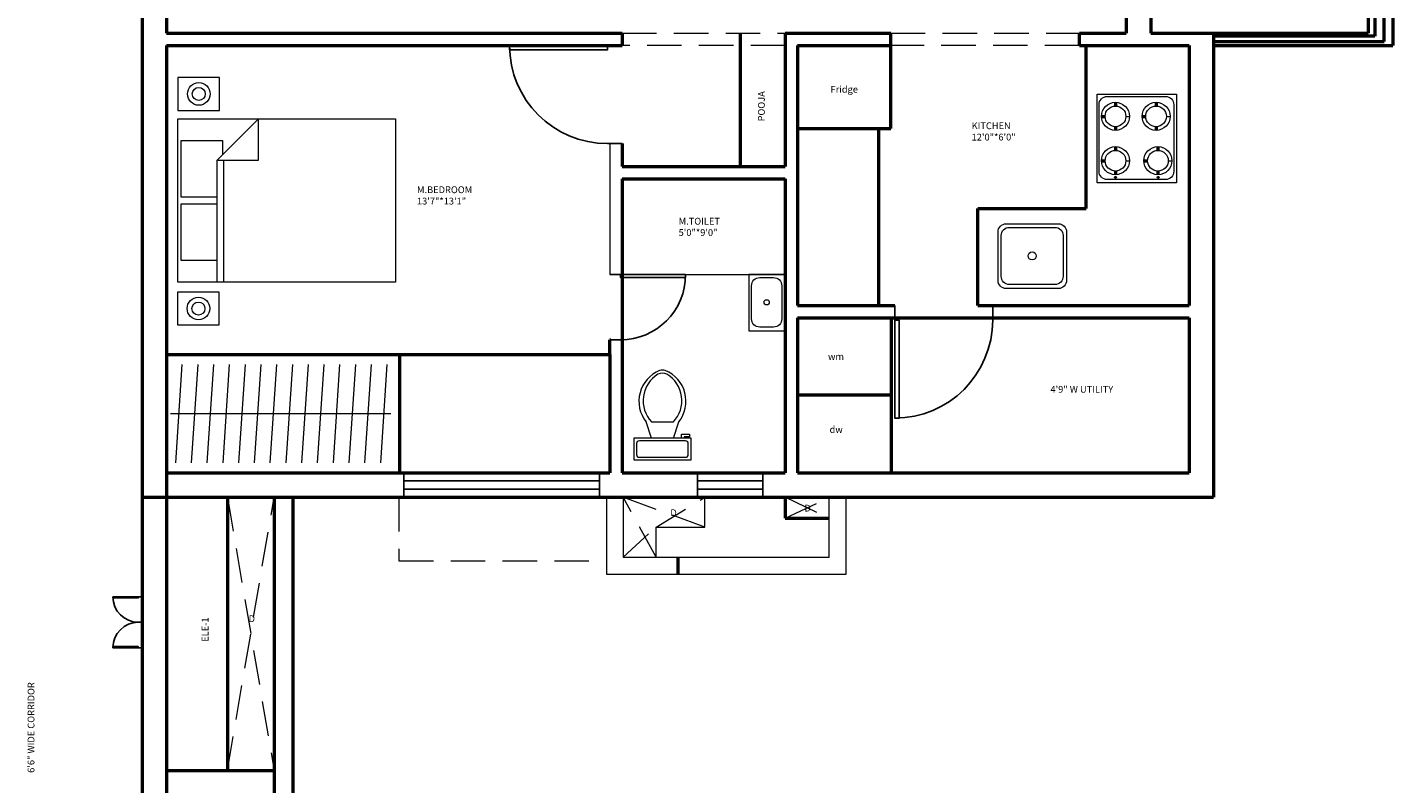
# Model space of a CAD drawing. Units: inches. Extents: x 4795 to 6024, y 2716 to 5025.
# Tile 15 of 19: x 5486 to 5988, y 3816 to 4094. Entities that reach past the tile are written whole.
import ezdxf

# ---------------------------------------------------------------- set-up
doc = ezdxf.new("R2010")
doc.units = ezdxf.units.IN
doc.linetypes.add('DASHED', pattern=[19.05, 12.7, -6.35])
for name, color, linetype, lineweight in [('A-ANNO-TEXT', 7, 'Continuous', 18), ('A-AREA-IDEN', 3, 'Continuous', 18), ('A-DOOR', 4, 'Continuous', 25), ('A-FLOR-FIXT', 9, 'Continuous', 18), ('A-FURN', 8, 'Continuous', 18), ('A-GLAZ', 4, 'Continuous', 25), ('A-WALL', 7, 'Continuous', 50), ('A-WALL-OVHD', 8, 'DASHED', 18)]:
    doc.layers.add(name, color=color, linetype=linetype, lineweight=lineweight)
doc.styles.get("Standard").update_dxf_attribs({"font": 'arial.ttf'})

# ---------------------------------------------------------------- blocks, each defined once
blk = doc.blocks.new('*U2')
for p, q in [((0, 0), (0, -6)), ((40, 0), (40, -6))]:
    blk.add_line(p, q)
blk.add_lwpolyline([(0, 0), (0, 40), (1.75, 40), (1.75, 0)], close=True)
blk.add_arc((0, 0), 40, 0, 90)
blk = doc.blocks.new('Bed - Queen')
for p, q in [((0, -80.00003), (0, 0)), ((0, 0), (59.99999, 0)), ((59.99999, 0), (59.99999, -80.00003)), ((7.99999, -1.2), (28.79998, -1.2)), ((7.99999, -14.4), (7.99999, -1.2)), ((28.79998, -1.2), (28.79998, -14.4)), ((31.19999, -1.2), (51.99999, -1.2)), ((31.19999, -14.4), (31.19999, -1.2)), ((51.99999, -1.2), (51.99999, -16.4)), ((0, -14.4), (44.8, -14.4)), ((59.99999, -29.6), (44.8, -14.4)), ((44.8, -14.4), (44.8, -29.6)), ((44.8, -16.8), (0, -16.8)), ((51.99999, -16.4), (46.79936, -16.4)), ((44.8, -29.6), (59.99999, -29.6)), ((59.99999, -80.00003), (0, -80.00003))]:
    blk.add_line(p, q)
blk = doc.blocks.new('Toilet - top')
for p, q in [((9.5, -6), (9.5, -2)), ((-10, -8.5), (-8, -8.5)), ((-10, -9.5), (-10, -8.5)), ((-7, -9.5), (-10, -9.5)), ((-8, -8.5), (-8, -8)), ((-7, -8), (-7, -9.5)), ((-4, -8), (-6, -14)), ((4, -8), (6, -14)), ((4, -14), (-4, -14))]:
    blk.add_line(p, q)
blk.add_lwpolyline([(10.5, -8), (10.5, 0), (-10.5, 0), (-10.5, -8)], close=True)
for points in [[(-9.5, -2), (-9.5, -6)], [(8.5, -1), (-8.5, -1)], [(-8.5, -7), (8.5, -7)]]:
    blk.add_lwpolyline(points)
for centre, radius, start, end in [((-8.62, -1.88), 0.884, 81.8699, 188.1301), ((8.62, -1.88), 0.884, 351.8699, 98.1301), ((-8.62, -6.12), 0.884, 171.8699, 278.1301), ((8.62, -6.12), 0.884, 261.8699, 8.1301), ((3.52, -21.58), 12.17, 141.4691, 247.9714), ((4.2, -21.82), 11.33, 136.3677, 238.9468), ((-3.52, -21.58), 12.17, 292.0284, 38.5307), ((-4.2, -21.82), 11.33, 301.053, 43.6321), ((0, -27.88), 4, 245.7318, 294.2682), ((0, -29), 4, 254.8605, 285.1395)]:
    blk.add_arc(centre, radius, start, end)
blk = doc.blocks.new('WIN-72')
for p, q in [((0, 0), (0, 9)), ((0, 9), (72, 9)), ((0, 6), (72, 6)), ((72, 9), (72, 0)), ((72, 3), (0, 3)), ((72, 0), (0, 0))]:
    blk.add_line(p, q)
blk = doc.blocks.new('WIN-24')
for p, q in [((0, 0), (0, 9)), ((0, 9), (24, 9)), ((0, 6), (24, 6)), ((24, 9), (24, 0)), ((24, 3), (0, 3)), ((24, 0), (0, 0))]:
    blk.add_line(p, q)

msp = doc.modelspace()

# ---------------------------------------------------------------- linework, layer by layer
at = {"layer": 'A-FLOR-FIXT'}
for points in [[(5879.38, 4068.91), (5908.62, 4068.91), (5908.62, 4036.39), (5879.38, 4036.39)], [(5764.72, 4002.66), (5751.28, 4002.66), (5751.28, 3981.93), (5764.72, 3981.93)]]:
    msp.add_lwpolyline(points, close=True, dxfattribs=at)
for points in [[(5883.1, 4068.11), (5904.57, 4068.11, -0.414214), (5907.57, 4065.11), (5907.57, 4040.56, -0.414214), (5904.57, 4037.56), (5883.1, 4037.56, -0.414214), (5880.1, 4040.56), (5880.1, 4065.11, -0.414214)], [(5845.95, 4021.32), (5865.16, 4021.32, -0.414214), (5868.16, 4018.32), (5868.16, 4000.52, -0.414214), (5865.16, 3997.52), (5845.95, 3997.52, -0.414214), (5842.95, 4000.52), (5842.95, 4018.32, -0.414214)], [(5847.15, 4020.01), (5863.88, 4020.01, -0.414214), (5866.88, 4017.01), (5866.88, 4001.99, -0.414214), (5863.88, 3998.99), (5847.15, 3998.99, -0.414214), (5844.15, 4001.99), (5844.15, 4017.01, -0.414214)], [(5755.32, 4001.56), (5760.43, 4001.56, -0.414214), (5763.43, 3998.56), (5763.43, 3986.34, -0.414214), (5760.43, 3983.34), (5755.32, 3983.34, -0.414214), (5752.32, 3986.34), (5752.32, 3998.56, -0.414214)]]:
    msp.add_lwpolyline(points, format="xyb", close=True, dxfattribs=at)
for centre, radius in [((5886.15, 4060.8), 5.16), ((5886.15, 4060.8), 3.8), ((5901.08, 4060.8), 5.16), ((5901.08, 4060.8), 3.8), ((5886.15, 4044.5), 5.16), ((5886.15, 4044.5), 3.8), ((5901.75, 4044.5), 5.16), ((5901.75, 4044.5), 3.8), ((5886.15, 4038.39), 0.353), ((5901.85, 4038.39), 0.353), ((5855.51, 4009.5), 1.48), ((5757.88, 3992.45), 0.951)]:
    msp.add_circle(centre, radius, dxfattribs=at)
at = {"layer": 'A-FURN'}
for p, q in [((5889.95, 4060.8), (5891.31, 4060.8)), ((5904.89, 4060.8), (5906.25, 4060.8)), ((5700.22, 4050.81), (5700.22, 4002.66)), ((5889.95, 4044.5), (5891.31, 4044.5)), ((5905.55, 4044.5), (5906.91, 4044.5)), ((5700.22, 4002.66), (5764.72, 4002.66)), ((5540.56, 3933.52), (5543, 3969.6)), ((5546.36, 3933.52), (5548.8, 3969.6)), ((5552.16, 3933.52), (5554.6, 3969.6)), ((5557.96, 3933.52), (5560.4, 3969.6)), ((5563.76, 3933.52), (5566.19, 3969.6)), ((5569.55, 3933.52), (5571.99, 3969.6)), ((5575.35, 3933.52), (5577.79, 3969.6)), ((5581.15, 3933.52), (5583.59, 3969.6)), ((5586.95, 3933.52), (5589.39, 3969.6)), ((5592.75, 3933.52), (5595.18, 3969.6)), ((5598.54, 3933.52), (5600.98, 3969.6)), ((5604.34, 3933.52), (5606.78, 3969.6)), ((5610.14, 3933.52), (5612.58, 3969.6)), ((5615.94, 3933.52), (5618.38, 3969.6)), ((5538.62, 3951.59), (5619.65, 3951.59)), ((5699.04, 3920.81), (5699.04, 3892.52)), ((5705.08, 3920.81), (5705.08, 3898.82)), ((5735.18, 3909.81), (5735.18, 3920.81)), ((5780.9, 3898.82), (5780.9, 3920.81)), ((5787.08, 3892.52), (5787.08, 3920.81)), ((5717.19, 3898.82), (5717.19, 3909.81)), ((5717.19, 3909.81), (5735.18, 3909.81)), ((5705.08, 3898.82), (5780.9, 3898.82)), ((5699.04, 3892.52), (5787.08, 3892.52))]:
    msp.add_line(p, q, dxfattribs=at)
for points in [[(5541.4, 4063.01), (5556.67, 4063.01), (5556.67, 4075.05), (5541.4, 4075.05)], [(5541.28, 3984.13), (5556.55, 3984.13), (5556.55, 3996.16), (5541.28, 3996.16)]]:
    msp.add_lwpolyline(points, close=True, dxfattribs=at)
for centre, radius in [((5549.04, 4069.03), 4.15), ((5549.04, 4069.03), 2.4), ((5548.91, 3990.15), 4.15), ((5548.91, 3990.15), 2.4)]:
    msp.add_circle(centre, radius, dxfattribs=at)
at = {"layer": 'A-WALL'}
for p, q in [((5528.22, 4507.98), (5528.22, 3920.81)), ((5988.09, 4227.81), (5988.09, 4086.81)), ((5537.22, 4223.31), (5537.22, 4091.31)), ((5890.09, 4223.31), (5890.09, 4091.31)), ((5899.09, 4223.31), (5899.09, 4091.31)), ((5979.09, 4223.31), (5979.09, 4091.31)), ((5981.57, 4223.31), (5981.57, 4090.21)), ((5984.99, 4088.3), (5984.99, 4223.31)), ((5537.22, 4091.31), (5704.72, 4091.31)), ((5704.72, 4091.31), (5704.72, 4086.81)), ((5748.18, 4091.31), (5748.18, 4042.31)), ((5764.72, 4091.31), (5764.72, 4042.31)), ((5764.72, 4091.31), (5803.49, 4091.31)), ((5803.49, 4056.32), (5803.49, 4091.31)), ((5872.89, 4086.76), (5872.89, 4091.31)), ((5872.89, 4091.31), (5890.09, 4091.31)), ((5899.09, 4091.31), (5922.22, 4091.31)), ((5922.22, 4091.31), (5922.22, 3920.81)), ((5922.22, 4091.31), (5979.09, 4091.31)), ((5981.57, 4090.21), (5922.22, 4090.21)), ((5922.22, 4088.3), (5984.99, 4088.3)), ((5537.22, 4086.81), (5704.72, 4086.81)), ((5537.22, 4086.81), (5537.22, 3929.81)), ((5769.22, 4086.81), (5769.22, 3991.31)), ((5769.22, 4086.81), (5803.49, 4086.81)), ((5872.89, 4086.81), (5913.22, 4086.81)), ((5875.33, 4026.93), (5875.33, 4086.81)), ((5913.22, 4086.81), (5913.22, 3991.31)), ((5922.22, 4086.81), (5988.09, 4086.81)), ((5886.15, 4065.96), (5886.15, 4064.61)), ((5901.08, 4065.96), (5901.08, 4064.61)), ((5880.99, 4060.8), (5882.35, 4060.8)), ((5886.15, 4057), (5886.15, 4055.64)), ((5895.92, 4060.8), (5897.28, 4060.8)), ((5901.08, 4057), (5901.08, 4055.64)), ((5769.22, 4056.32), (5798.96, 4056.32)), ((5798.96, 4056.32), (5798.96, 3991.31)), ((5798.96, 4056.32), (5803.49, 4056.32)), ((5704.72, 4050.81), (5704.72, 4042.31)), ((5886.15, 4049.66), (5886.15, 4048.3)), ((5901.75, 4049.66), (5901.75, 4048.3)), ((5704.72, 4042.31), (5764.72, 4042.31)), ((5880.99, 4044.5), (5882.35, 4044.5)), ((5896.58, 4044.5), (5897.94, 4044.5)), ((5704.72, 4037.81), (5764.72, 4037.81)), ((5704.72, 4037.81), (5704.72, 3929.81)), ((5764.72, 4037.81), (5764.72, 3929.81)), ((5886.15, 4040.69), (5886.15, 4039.33)), ((5901.75, 4040.69), (5901.75, 4039.33)), ((5835.54, 3991.31), (5835.54, 4026.93)), ((5835.54, 4026.93), (5875.33, 4026.93)), ((5769.22, 3991.31), (5804.99, 3991.31)), ((5769.22, 3986.81), (5913.22, 3986.81)), ((5769.22, 3986.81), (5769.22, 3929.81)), ((5803.71, 3986.81), (5803.71, 3929.81)), ((5835.54, 3991.31), (5913.22, 3991.31)), ((5913.22, 3986.81), (5913.22, 3929.81)), ((5700.22, 3973.3), (5700.22, 3978.66)), ((5700.48, 3978.66), (5700.22, 3978.66)), ((5537.22, 3973.3), (5700.22, 3973.3)), ((5622.92, 3973.3), (5622.92, 3929.81)), ((5700.22, 3973.3), (5700.22, 3929.81)), ((5803.71, 3958.31), (5769.22, 3958.31)), ((5537.22, 3929.81), (5700.22, 3929.81)), ((5537.22, 3929.81), (5537.22, 3740.43)), ((5704.72, 3929.81), (5764.72, 3929.81)), ((5769.22, 3929.81), (5913.22, 3929.81)), ((5528.22, 3920.81), (5922.22, 3920.81)), ((5528.22, 3920.81), (5528.22, 3351.93)), ((5559.58, 3920.81), (5559.58, 3820.38)), ((5576.74, 3920.81), (5576.74, 3740.43)), ((5583.63, 3920.81), (5583.63, 3740.43)), ((5764.72, 3920.81), (5764.72, 3913.08)), ((5764.72, 3913.08), (5780.9, 3913.08)), ((5725.18, 3898.82), (5725.18, 3892.52)), ((5537.22, 3820.38), (5576.74, 3820.38))]:
    msp.add_line(p, q, dxfattribs=at)
at = {"layer": 'A-WALL-OVHD'}
for p, q in [((5704.72, 4091.31), (5764.72, 4091.31)), ((5803.49, 4091.31), (5872.89, 4091.31)), ((5764.72, 4086.81), (5704.72, 4086.81)), ((5872.89, 4086.81), (5803.49, 4086.81)), ((5559.58, 3920.81), (5576.74, 3820.38)), ((5559.58, 3820.38), (5576.74, 3920.81)), ((5622.65, 3920.91), (5622.65, 3897.46)), ((5717.19, 3898.82), (5705.08, 3920.81)), ((5735.18, 3909.81), (5705.18, 3920.81)), ((5717.19, 3909.81), (5735.18, 3920.81)), ((5764.72, 3920.81), (5764.79, 3920.81)), ((5764.72, 3913.08), (5780.9, 3920.81)), ((5764.79, 3920.81), (5780.9, 3913.08)), ((5705.08, 3898.82), (5717.19, 3909.81)), ((5622.65, 3897.46), (5699.04, 3897.46))]:
    msp.add_line(p, q, dxfattribs=at)

# ---------------------------------------------------------------- block references
at = {"layer": 'A-DOOR'}
for p, xscale, yscale, zscale, rotation in [((5699.32, 4086.81), -0.9, 0.9, 0.9, 90), ((5704.08, 4002.66), 0.6, 0.6, 0.6, 270), ((5804.99, 3985.91), -0.9, 0.9, 0.9, 180), ((5526.82, 3884.21), -0.2337145210718518, 0.2337145210718518, 0.2337145210718518, 90), ((5526.82, 3865.51), 0.2337145210718518, 0.2337145210718518, 0.2337145210718518, 89.99999999999999)]:
    msp.add_blockref('*U2', p, dxfattribs=dict(at, xscale=xscale, yscale=yscale, zscale=zscale, rotation=rotation))
at = {"layer": 'A-FLOR-FIXT', "rotation": 180}
msp.add_blockref('Toilet - top', (5719.56, 3934.51), dxfattribs=at)
at = {"layer": 'A-FURN', "rotation": 90}
msp.add_blockref('Bed - Queen', (5541.37, 3999.88), dxfattribs=at)
at = {"layer": 'A-GLAZ', "rotation": 180}
for name, p in [('WIN-72', (5696.43, 3929.81)), ('WIN-24', (5756.48, 3929.81))]:
    msp.add_blockref(name, p, dxfattribs=at)

# ---------------------------------------------------------------- texts
at = {"layer": 'A-ANNO-TEXT', "char_height": 2.5, "attachment_point": 1}
for s, width, insert in [('Fridge', 19.5033, (5781.37, 4071.99)), ('wm', 14.5317, (5780.44, 3973.79)), ('dw', 12.4602, (5781.01, 3946.97)), ('D', 2.1996, (5722.47, 3916.37)), ('D', 2.067, (5771.75, 3918.06)), ('D', 1.088, (5567.38, 3877.41))]:
    msp.add_mtext_dynamic_manual_height_columns(s, width=width, gutter_width=12.5, heights=[0], dxfattribs=dict(at, insert=insert))
at = {"layer": 'A-ANNO-TEXT', "insert": (5550.13, 3867.7), "char_height": 2.5, "attachment_point": 1, "rotation": 90}
msp.add_mtext_dynamic_manual_height_columns('ELE-1', width=16.7049, gutter_width=12.5, heights=[0], dxfattribs=at)
at = {"layer": 'A-AREA-IDEN', "char_height": 2.5, "attachment_point": 1, "rotation": 90}
for s, width, insert in [('POOJA', 11.2346, (5754.7, 4058.93)), ('6\'6" WIDE CORRIDOR', 60.1936, (5486.12, 3819.52))]:
    msp.add_mtext_dynamic_manual_height_columns(s, width=width, gutter_width=12.5, heights=[0], dxfattribs=dict(at, insert=insert))
at = {"layer": 'A-AREA-IDEN', "char_height": 2.5, "attachment_point": 1}
for s, width, insert in [('KITCHEN\\P12\'0"*6\'0"', 47.2466, (5833.25, 4058.59)), ('M.BEDROOM\\P13\'7"*13\'1"', 58.2267, (5629.29, 4035.07)), ('M.TOILET\\P5\'0"*9\'0"', 41.9189, (5725.5, 4023.51)), ('4\'9" W UTILITY', 53.9793, (5862.23, 3961.73))]:
    msp.add_mtext_dynamic_manual_height_columns(s, width=width, gutter_width=12.5, heights=[0], dxfattribs=dict(at, insert=insert))

doc.saveas('drawing.dxf')
